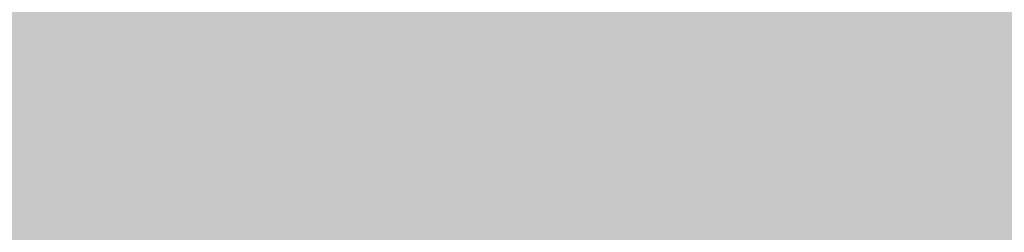
# Model space of a CAD drawing. Units: millimetres. Extents: x -22994 to 29398, y -19990 to 20176.
# Tile 75 of 135: x 226.355 to 227.437, y 84.264 to 84.498. Entities that reach past the tile are written whole.
import ezdxf
from ezdxf import colors
from ezdxf.entities.mleader import LeaderData, LeaderLine
from ezdxf.math import Vec2, Vec3

# ---------------------------------------------------------------- set-up
doc = ezdxf.new("R2010")
doc.units = ezdxf.units.MM
doc.header["$MEASUREMENT"] = 0
for name, color, linetype, lineweight in [('M-ANNO-TEXT', 7, 'Continuous', 25), ('M-DIMS', 2, 'Continuous', 18), ('M-EQPM-PATT', 7, 'Continuous', 18)]:
    doc.layers.add(name, color=color, linetype=linetype, lineweight=lineweight)
doc.styles.get("Standard").update_dxf_attribs({"font": 'arial.ttf'})
doc.dimstyles.get("Standard").update_dxf_attribs({"dimtxt": 0.18, "dimasz": 10000, "dimexe": 0.18, "dimexo": 0.0625, "dimgap": 0.09, "dimtad": 0, "dimtih": 1, "dimtoh": 1, "dimdec": 0, "dimzin": 0, "dimdsep": 46, "dimtxsty": 'Standard', "dimcen": 0.09, "dimadec": 0, "dimazin": 0, "dimtfac": 1, "dimtdec": 0, "dimtofl": 0, "dimtmove": 0, "dimatfit": 3, "dimfxl": 1, "dimtolj": 1, "dimtzin": 0, "dimlwd": 30, "dimarcsym": 0})

# ---------------------------------------------------------------- blocks, each defined once
blk = doc.blocks.new('*D2')
at = {"layer": 'Defpoints', "color": 0, "transparency": 16777216}
for p in [(6.6773, 10.2713), (290.852, 10.2713), (290.852, -5.0787)]:
    blk.add_point(p, dxfattribs=at)
at = {"layer": 'M-DIMS', "color": 0, "lineweight": -2, "transparency": 16777216}
for p, q in [((6.6773, 10.2088), (6.6773, -5.2587)), ((290.852, 10.2088), (290.852, -5.2587))]:
    blk.add_line(p, q, dxfattribs=at)
at = {"layer": 'M-DIMS', "color": 0, "lineweight": 30, "transparency": 16777216}
for p, q in [((-9993.3227, -5.0787), (-19993.3227, -5.0787)), ((10290.852, -5.0787), (20290.852, -5.0787))]:
    blk.add_line(p, q, dxfattribs=at)
at = {"layer": 'M-DIMS', "color": 0, "transparency": 16777216}
for points in [[(-9993.3227, 1661.5879), (-9993.3227, -1671.7454), (6.6773, -5.0787)], [(10290.852, 1661.5879), (10290.852, -1671.7454), (290.852, -5.0787)]]:
    blk.add_solid(points, dxfattribs=at)
at = {"layer": 'M-DIMS', "color": 0, "transparency": 16777216, "insert": (148.7647, -5.0787), "char_height": 0.18, "attachment_point": 5}
blk.add_mtext('\\A1;284.2', dxfattribs=at)
blk = doc.blocks.new('*D3')
at = {"layer": 'Defpoints', "color": 0, "transparency": 16777216}
for p in [(110.2647, 204.1654), (110.2647, 176.3662), (95.8327, 127.967)]:
    blk.add_point(p, dxfattribs=at)
at = {"layer": 'M-DIMS', "color": 0, "lineweight": -2, "transparency": 16777216}
for p, q in [((95.8327, 128.0295), (95.8327, 204.3454)), ((110.2647, 176.4287), (110.2647, 204.3454))]:
    blk.add_line(p, q, dxfattribs=at)
at = {"layer": 'M-DIMS', "color": 0, "lineweight": 30, "transparency": 16777216}
for p, q in [((-9904.1673, 204.1654), (-19904.1673, 204.1654)), ((10110.2647, 204.1654), (20110.2647, 204.1654))]:
    blk.add_line(p, q, dxfattribs=at)
at = {"layer": 'M-DIMS', "color": 0, "transparency": 16777216}
for points in [[(-9904.1673, 1870.8321), (-9904.1673, -1462.5013), (95.8327, 204.1654)], [(10110.2647, 1870.8321), (10110.2647, -1462.5013), (110.2647, 204.1654)]]:
    blk.add_solid(points, dxfattribs=at)
at = {"layer": 'M-DIMS', "color": 0, "transparency": 16777216, "insert": (103.0487, 204.1654), "char_height": 0.18, "attachment_point": 5}
blk.add_mtext('\\A1;14.432', dxfattribs=at)
blk = doc.blocks.new('*D4')
at = {"layer": 'Defpoints', "color": 0, "transparency": 16777216}
for p in [(116.2647, 204.1654), (110.2647, 176.3662), (116.2647, 176.3662)]:
    blk.add_point(p, dxfattribs=at)
at = {"layer": 'M-DIMS', "color": 0, "lineweight": -2, "transparency": 16777216}
for p, q in [((110.2647, 176.4287), (110.2647, 204.3454)), ((116.2647, 176.4287), (116.2647, 204.3454))]:
    blk.add_line(p, q, dxfattribs=at)
at = {"layer": 'M-DIMS', "color": 0, "lineweight": 30, "transparency": 16777216}
for p, q in [((-9889.7353, 204.1654), (-19889.7353, 204.1654)), ((10116.2647, 204.1654), (20116.2647, 204.1654))]:
    blk.add_line(p, q, dxfattribs=at)
at = {"layer": 'M-DIMS', "color": 0, "transparency": 16777216}
for points in [[(-9889.7353, 1870.8321), (-9889.7353, -1462.5013), (110.2647, 204.1654)], [(10116.2647, 1870.8321), (10116.2647, -1462.5013), (116.2647, 204.1654)]]:
    blk.add_solid(points, dxfattribs=at)
at = {"layer": 'M-DIMS', "color": 0, "transparency": 16777216, "insert": (113.2647, 204.1654), "char_height": 0.18, "attachment_point": 5}
blk.add_mtext('\\A1;6', dxfattribs=at)
blk = doc.blocks.new('*D5')
at = {"layer": 'Defpoints', "color": 0, "transparency": 16777216}
for p in [(181.2647, 204.1654), (116.2647, 176.3662), (181.2647, 176.3662)]:
    blk.add_point(p, dxfattribs=at)
at = {"layer": 'M-DIMS', "color": 0, "lineweight": -2, "transparency": 16777216}
for p, q in [((116.2647, 176.4287), (116.2647, 204.3454)), ((181.2647, 176.4287), (181.2647, 204.3454))]:
    blk.add_line(p, q, dxfattribs=at)
at = {"layer": 'M-DIMS', "color": 0, "lineweight": 30, "transparency": 16777216}
for p, q in [((-9883.7353, 204.1654), (-19883.7353, 204.1654)), ((10181.2647, 204.1654), (20181.2647, 204.1654))]:
    blk.add_line(p, q, dxfattribs=at)
at = {"layer": 'M-DIMS', "color": 0, "transparency": 16777216}
for points in [[(-9883.7353, 1870.8321), (-9883.7353, -1462.5013), (116.2647, 204.1654)], [(10181.2647, 1870.8321), (10181.2647, -1462.5013), (181.2647, 204.1654)]]:
    blk.add_solid(points, dxfattribs=at)
at = {"layer": 'M-DIMS', "color": 0, "transparency": 16777216, "insert": (148.7647, 204.1654), "char_height": 0.18, "attachment_point": 5}
blk.add_mtext('\\A1;65', dxfattribs=at)
blk = doc.blocks.new('*D6')
at = {"layer": 'Defpoints', "color": 0, "transparency": 16777216}
for p in [(187.2647, 204.1654), (181.2647, 176.3662), (187.2647, 176.3662)]:
    blk.add_point(p, dxfattribs=at)
at = {"layer": 'M-DIMS', "color": 0, "lineweight": -2, "transparency": 16777216}
for p, q in [((181.2647, 176.4287), (181.2647, 204.3454)), ((187.2647, 176.4287), (187.2647, 204.3454))]:
    blk.add_line(p, q, dxfattribs=at)
at = {"layer": 'M-DIMS', "color": 0, "lineweight": 30, "transparency": 16777216}
for p, q in [((-9818.7353, 204.1654), (-19818.7353, 204.1654)), ((10187.2647, 204.1654), (20187.2647, 204.1654))]:
    blk.add_line(p, q, dxfattribs=at)
at = {"layer": 'M-DIMS', "color": 0, "transparency": 16777216}
for points in [[(-9818.7353, 1870.8321), (-9818.7353, -1462.5013), (181.2647, 204.1654)], [(10187.2647, 1870.8321), (10187.2647, -1462.5013), (187.2647, 204.1654)]]:
    blk.add_solid(points, dxfattribs=at)
at = {"layer": 'M-DIMS', "color": 0, "transparency": 16777216, "insert": (184.2647, 204.1654), "char_height": 0.18, "attachment_point": 5}
blk.add_mtext('\\A1;6', dxfattribs=at)
blk = doc.blocks.new('*D7')
at = {"layer": 'Defpoints', "color": 0, "transparency": 16777216}
for p in [(201.6967, 204.1654), (187.2647, 176.3662), (201.6967, 127.967)]:
    blk.add_point(p, dxfattribs=at)
at = {"layer": 'M-DIMS', "color": 0, "lineweight": -2, "transparency": 16777216}
for p, q in [((187.2647, 176.4287), (187.2647, 204.3454)), ((201.6967, 128.0295), (201.6967, 204.3454))]:
    blk.add_line(p, q, dxfattribs=at)
at = {"layer": 'M-DIMS', "color": 0, "lineweight": 30, "transparency": 16777216}
for p, q in [((-9812.7353, 204.1654), (-19812.7353, 204.1654)), ((10201.6967, 204.1654), (20201.6967, 204.1654))]:
    blk.add_line(p, q, dxfattribs=at)
at = {"layer": 'M-DIMS', "color": 0, "transparency": 16777216}
for points in [[(-9812.7353, 1870.8321), (-9812.7353, -1462.5013), (187.2647, 204.1654)], [(10201.6967, 1870.8321), (10201.6967, -1462.5013), (201.6967, 204.1654)]]:
    blk.add_solid(points, dxfattribs=at)
at = {"layer": 'M-DIMS', "color": 0, "transparency": 16777216, "insert": (194.4807, 204.1654), "char_height": 0.18, "attachment_point": 5}
blk.add_mtext('\\A1;14.432', dxfattribs=at)
blk = doc.blocks.new('*D8')
at = {"layer": 'Defpoints', "color": 0, "transparency": 16777216}
for p in [(227.6485, 204.1654), (227.6485, 146.7296), (201.6967, 127.967)]:
    blk.add_point(p, dxfattribs=at)
at = {"layer": 'M-DIMS', "color": 0, "lineweight": -2, "transparency": 16777216}
for p, q in [((201.6967, 128.0295), (201.6967, 204.3454)), ((227.6485, 146.7921), (227.6485, 204.3454))]:
    blk.add_line(p, q, dxfattribs=at)
at = {"layer": 'M-DIMS', "color": 0, "lineweight": 30, "transparency": 16777216}
for p, q in [((-9798.3033, 204.1654), (-19798.3033, 204.1654)), ((10227.6485, 204.1654), (20227.6485, 204.1654))]:
    blk.add_line(p, q, dxfattribs=at)
at = {"layer": 'M-DIMS', "color": 0, "transparency": 16777216}
for points in [[(-9798.3033, 1870.8321), (-9798.3033, -1462.5013), (201.6967, 204.1654)], [(10227.6485, 1870.8321), (10227.6485, -1462.5013), (227.6485, 204.1654)]]:
    blk.add_solid(points, dxfattribs=at)
at = {"layer": 'M-DIMS', "color": 0, "transparency": 16777216, "insert": (214.6726, 204.1654), "char_height": 0.18, "attachment_point": 5}
blk.add_mtext('\\A1;25.95', dxfattribs=at)
blk = doc.blocks.new('*D9')
at = {"layer": 'Defpoints', "color": 0, "transparency": 16777216}
for p in [(187.2647, 176.3662), (306.202, 176.3662), (290.852, 10.2713)]:
    blk.add_point(p, dxfattribs=at)
at = {"layer": 'M-DIMS', "color": 0, "lineweight": 30, "transparency": 16777216}
for p, q in [((306.202, 10176.3662), (306.202, 20176.3662)), ((306.202, -9989.7287), (306.202, -19989.7287))]:
    blk.add_line(p, q, dxfattribs=at)
at = {"layer": 'M-DIMS', "color": 0, "lineweight": -2, "transparency": 16777216}
for p, q in [((187.3272, 176.3662), (306.382, 176.3662)), ((290.9145, 10.2713), (306.382, 10.2713))]:
    blk.add_line(p, q, dxfattribs=at)
at = {"layer": 'M-DIMS', "color": 0, "transparency": 16777216}
for points in [[(-1360.4646, 10176.3662), (1972.8687, 10176.3662), (306.202, 176.3662)], [(-1360.4646, -9989.7287), (1972.8687, -9989.7287), (306.202, 10.2713)]]:
    blk.add_solid(points, dxfattribs=at)
at = {"layer": 'M-DIMS', "color": 0, "transparency": 16777216, "insert": (306.202, 93.3187), "char_height": 0.18, "attachment_point": 5}
blk.add_mtext('\\A1;166.1', dxfattribs=at)
blk = doc.blocks.new('*D10')
at = {"layer": 'Defpoints', "color": 0, "transparency": 16777216}
for p in [(125.6498, 136.0713), (133.3459, 136.0713), (133.3459, -5.0787)]:
    blk.add_point(p, dxfattribs=at)
at = {"layer": 'M-DIMS', "color": 0, "lineweight": -2, "transparency": 16777216}
for p, q in [((125.6498, 136.0088), (125.6498, -5.2587)), ((133.3459, 136.0088), (133.3459, -5.2587))]:
    blk.add_line(p, q, dxfattribs=at)
at = {"layer": 'M-DIMS', "color": 0, "lineweight": 30, "transparency": 16777216}
for p, q in [((-9874.3502, -5.0787), (-19874.3502, -5.0787)), ((10133.3459, -5.0787), (20133.3459, -5.0787))]:
    blk.add_line(p, q, dxfattribs=at)
at = {"layer": 'M-DIMS', "color": 0, "transparency": 16777216}
for points in [[(-9874.3502, 1661.5879), (-9874.3502, -1671.7454), (125.6498, -5.0787)], [(10133.3459, 1661.5879), (10133.3459, -1671.7454), (133.3459, -5.0787)]]:
    blk.add_solid(points, dxfattribs=at)
at = {"layer": 'M-DIMS', "color": 0, "transparency": 16777216, "insert": (129.4978, -5.0787), "char_height": 0.18, "attachment_point": 5}
blk.add_mtext('\\A1;7.696', dxfattribs=at)
blk = doc.blocks.new('*D11')
at = {"layer": 'Defpoints', "color": 0, "transparency": 16777216}
for p in [(133.3459, 136.0713), (135.6498, 136.0713), (135.6498, -5.0787)]:
    blk.add_point(p, dxfattribs=at)
at = {"layer": 'M-DIMS', "color": 0, "lineweight": -2, "transparency": 16777216}
for p, q in [((133.3459, 136.0088), (133.3459, -5.2587)), ((135.6498, 136.0088), (135.6498, -5.2587))]:
    blk.add_line(p, q, dxfattribs=at)
at = {"layer": 'M-DIMS', "color": 0, "lineweight": 30, "transparency": 16777216}
for p, q in [((-9866.6541, -5.0787), (-19866.6541, -5.0787)), ((10135.6498, -5.0787), (20135.6498, -5.0787))]:
    blk.add_line(p, q, dxfattribs=at)
at = {"layer": 'M-DIMS', "color": 0, "transparency": 16777216}
for points in [[(-9866.6541, 1661.5879), (-9866.6541, -1671.7454), (133.3459, -5.0787)], [(10135.6498, 1661.5879), (10135.6498, -1671.7454), (135.6498, -5.0787)]]:
    blk.add_solid(points, dxfattribs=at)
at = {"layer": 'M-DIMS', "color": 0, "transparency": 16777216, "insert": (134.4978, -5.0787), "char_height": 0.18, "attachment_point": 5}
blk.add_mtext('\\A1;2.304', dxfattribs=at)
blk = doc.blocks.new('*D12')
at = {"layer": 'Defpoints', "color": 0, "transparency": 16777216}
for p in [(135.6498, 136.0713), (145.6498, 136.0713), (145.6498, -5.0787)]:
    blk.add_point(p, dxfattribs=at)
at = {"layer": 'M-DIMS', "color": 0, "lineweight": -2, "transparency": 16777216}
for p, q in [((135.6498, 136.0088), (135.6498, -5.2587)), ((145.6498, 136.0088), (145.6498, -5.2587))]:
    blk.add_line(p, q, dxfattribs=at)
at = {"layer": 'M-DIMS', "color": 0, "lineweight": 30, "transparency": 16777216}
for p, q in [((-9864.3502, -5.0787), (-19864.3502, -5.0787)), ((10145.6498, -5.0787), (20145.6498, -5.0787))]:
    blk.add_line(p, q, dxfattribs=at)
at = {"layer": 'M-DIMS', "color": 0, "transparency": 16777216}
for points in [[(-9864.3502, 1661.5879), (-9864.3502, -1671.7454), (135.6498, -5.0787)], [(10145.6498, 1661.5879), (10145.6498, -1671.7454), (145.6498, -5.0787)]]:
    blk.add_solid(points, dxfattribs=at)
at = {"layer": 'M-DIMS', "color": 0, "transparency": 16777216, "insert": (140.6498, -5.0787), "char_height": 0.18, "attachment_point": 5}
blk.add_mtext('\\A1;10', dxfattribs=at)
blk = doc.blocks.new('*D13')
at = {"layer": 'Defpoints', "color": 0, "transparency": 16777216}
for p in [(145.6498, 136.0713), (155.6498, 136.0713), (155.6498, -5.0787)]:
    blk.add_point(p, dxfattribs=at)
at = {"layer": 'M-DIMS', "color": 0, "lineweight": -2, "transparency": 16777216}
for p, q in [((145.6498, 136.0088), (145.6498, -5.2587)), ((155.6498, 136.0088), (155.6498, -5.2587))]:
    blk.add_line(p, q, dxfattribs=at)
at = {"layer": 'M-DIMS', "color": 0, "lineweight": 30, "transparency": 16777216}
for p, q in [((-9854.3502, -5.0787), (-19854.3502, -5.0787)), ((10155.6498, -5.0787), (20155.6498, -5.0787))]:
    blk.add_line(p, q, dxfattribs=at)
at = {"layer": 'M-DIMS', "color": 0, "transparency": 16777216}
for points in [[(-9854.3502, 1661.5879), (-9854.3502, -1671.7454), (145.6498, -5.0787)], [(10155.6498, 1661.5879), (10155.6498, -1671.7454), (155.6498, -5.0787)]]:
    blk.add_solid(points, dxfattribs=at)
at = {"layer": 'M-DIMS', "color": 0, "transparency": 16777216, "insert": (150.6498, -5.0787), "char_height": 0.18, "attachment_point": 5}
blk.add_mtext('\\A1;10', dxfattribs=at)
blk = doc.blocks.new('*D14')
at = {"layer": 'Defpoints', "color": 0, "transparency": 16777216}
for p in [(155.6498, 136.0713), (165.6498, 136.0713), (165.6498, -5.0787)]:
    blk.add_point(p, dxfattribs=at)
at = {"layer": 'M-DIMS', "color": 0, "lineweight": -2, "transparency": 16777216}
for p, q in [((155.6498, 136.0088), (155.6498, -5.2587)), ((165.6498, 136.0088), (165.6498, -5.2587))]:
    blk.add_line(p, q, dxfattribs=at)
at = {"layer": 'M-DIMS', "color": 0, "lineweight": 30, "transparency": 16777216}
for p, q in [((-9844.3502, -5.0787), (-19844.3502, -5.0787)), ((10165.6498, -5.0787), (20165.6498, -5.0787))]:
    blk.add_line(p, q, dxfattribs=at)
at = {"layer": 'M-DIMS', "color": 0, "transparency": 16777216}
for points in [[(-9844.3502, 1661.5879), (-9844.3502, -1671.7454), (155.6498, -5.0787)], [(10165.6498, 1661.5879), (10165.6498, -1671.7454), (165.6498, -5.0787)]]:
    blk.add_solid(points, dxfattribs=at)
at = {"layer": 'M-DIMS', "color": 0, "transparency": 16777216, "insert": (160.6498, -5.0787), "char_height": 0.18, "attachment_point": 5}
blk.add_mtext('\\A1;10', dxfattribs=at)
blk = doc.blocks.new('*D15')
at = {"layer": 'Defpoints', "color": 0, "transparency": 16777216}
for p in [(173.3459, 154.788), (173.3459, 136.0713), (306.202, 136.0713)]:
    blk.add_point(p, dxfattribs=at)
at = {"layer": 'M-DIMS', "color": 0, "lineweight": 30, "transparency": 16777216}
for p, q in [((306.202, 10154.788), (306.202, 20154.788)), ((306.202, -9863.9287), (306.202, -19863.9287))]:
    blk.add_line(p, q, dxfattribs=at)
at = {"layer": 'M-DIMS', "color": 0, "lineweight": -2, "transparency": 16777216}
for p, q in [((173.4084, 154.788), (306.382, 154.788)), ((173.4084, 136.0713), (306.382, 136.0713))]:
    blk.add_line(p, q, dxfattribs=at)
at = {"layer": 'M-DIMS', "color": 0, "transparency": 16777216}
for points in [[(-1360.4646, 10154.788), (1972.8687, 10154.788), (306.202, 154.788)], [(-1360.4646, -9863.9287), (1972.8687, -9863.9287), (306.202, 136.0713)]]:
    blk.add_solid(points, dxfattribs=at)
at = {"layer": 'M-DIMS', "color": 0, "transparency": 16777216, "insert": (306.202, 145.4297), "char_height": 0.18, "attachment_point": 5}
blk.add_mtext('\\A1;18.717', dxfattribs=at)
blk = doc.blocks.new('*D16')
at = {"layer": 'Defpoints', "color": 0, "transparency": 16777216}
for p in [(120.1702, 204.1654), (110.4658, 48.0349), (120.1702, 48.0349)]:
    blk.add_point(p, dxfattribs=at)
at = {"layer": 'M-DIMS', "color": 0, "lineweight": -2, "transparency": 16777216}
for p, q in [((110.4658, 48.0974), (110.4658, 204.3454)), ((120.1702, 48.0974), (120.1702, 204.3454))]:
    blk.add_line(p, q, dxfattribs=at)
at = {"layer": 'M-DIMS', "color": 0, "lineweight": 30, "transparency": 16777216}
for p, q in [((-9889.5342, 204.1654), (-19889.5342, 204.1654)), ((10120.1702, 204.1654), (20120.1702, 204.1654))]:
    blk.add_line(p, q, dxfattribs=at)
at = {"layer": 'M-DIMS', "color": 0, "transparency": 16777216}
for points in [[(-9889.5342, 1870.8321), (-9889.5342, -1462.5013), (110.4658, 204.1654)], [(10120.1702, 1870.8321), (10120.1702, -1462.5013), (120.1702, 204.1654)]]:
    blk.add_solid(points, dxfattribs=at)
at = {"layer": 'M-DIMS', "color": 0, "transparency": 16777216, "insert": (115.318, 204.1654), "char_height": 0.18, "attachment_point": 5}
blk.add_mtext('\\A1;9.704', dxfattribs=at)
blk = doc.blocks.new('*D17')
at = {"layer": 'Defpoints', "color": 0, "transparency": 16777216}
for p in [(126.1702, 204.1654), (120.1702, 48.0349), (126.1702, 48.0349)]:
    blk.add_point(p, dxfattribs=at)
at = {"layer": 'M-DIMS', "color": 0, "lineweight": -2, "transparency": 16777216}
for p, q in [((120.1702, 48.0974), (120.1702, 204.3454)), ((126.1702, 48.0974), (126.1702, 204.3454))]:
    blk.add_line(p, q, dxfattribs=at)
at = {"layer": 'M-DIMS', "color": 0, "lineweight": 30, "transparency": 16777216}
for p, q in [((-9879.8298, 204.1654), (-19879.8298, 204.1654)), ((10126.1702, 204.1654), (20126.1702, 204.1654))]:
    blk.add_line(p, q, dxfattribs=at)
at = {"layer": 'M-DIMS', "color": 0, "transparency": 16777216}
for points in [[(-9879.8298, 1870.8321), (-9879.8298, -1462.5013), (120.1702, 204.1654)], [(10126.1702, 1870.8321), (10126.1702, -1462.5013), (126.1702, 204.1654)]]:
    blk.add_solid(points, dxfattribs=at)
at = {"layer": 'M-DIMS', "color": 0, "transparency": 16777216, "insert": (123.1702, 204.1654), "char_height": 0.18, "attachment_point": 5}
blk.add_mtext('\\A1;6', dxfattribs=at)
blk = doc.blocks.new('*D18')
at = {"layer": 'Defpoints', "color": 0, "transparency": 16777216}
for p in [(132.1702, 204.1654), (126.1702, 48.0349), (132.1702, 48.0349)]:
    blk.add_point(p, dxfattribs=at)
at = {"layer": 'M-DIMS', "color": 0, "lineweight": -2, "transparency": 16777216}
for p, q in [((126.1702, 48.0974), (126.1702, 204.3454)), ((132.1702, 48.0974), (132.1702, 204.3454))]:
    blk.add_line(p, q, dxfattribs=at)
at = {"layer": 'M-DIMS', "color": 0, "lineweight": 30, "transparency": 16777216}
for p, q in [((-9873.8298, 204.1654), (-19873.8298, 204.1654)), ((10132.1702, 204.1654), (20132.1702, 204.1654))]:
    blk.add_line(p, q, dxfattribs=at)
at = {"layer": 'M-DIMS', "color": 0, "transparency": 16777216}
for points in [[(-9873.8298, 1870.8321), (-9873.8298, -1462.5013), (126.1702, 204.1654)], [(10132.1702, 1870.8321), (10132.1702, -1462.5013), (132.1702, 204.1654)]]:
    blk.add_solid(points, dxfattribs=at)
at = {"layer": 'M-DIMS', "color": 0, "transparency": 16777216, "insert": (129.1702, 204.1654), "char_height": 0.18, "attachment_point": 5}
blk.add_mtext('\\A1;6', dxfattribs=at)
blk = doc.blocks.new('*D19')
at = {"layer": 'Defpoints', "color": 0, "transparency": 16777216}
for p in [(138.1702, 204.1654), (132.1702, 48.0349), (138.1702, 48.0349)]:
    blk.add_point(p, dxfattribs=at)
at = {"layer": 'M-DIMS', "color": 0, "lineweight": -2, "transparency": 16777216}
for p, q in [((132.1702, 48.0974), (132.1702, 204.3454)), ((138.1702, 48.0974), (138.1702, 204.3454))]:
    blk.add_line(p, q, dxfattribs=at)
at = {"layer": 'M-DIMS', "color": 0, "lineweight": 30, "transparency": 16777216}
for p, q in [((-9867.8298, 204.1654), (-19867.8298, 204.1654)), ((10138.1702, 204.1654), (20138.1702, 204.1654))]:
    blk.add_line(p, q, dxfattribs=at)
at = {"layer": 'M-DIMS', "color": 0, "transparency": 16777216}
for points in [[(-9867.8298, 1870.8321), (-9867.8298, -1462.5013), (132.1702, 204.1654)], [(10138.1702, 1870.8321), (10138.1702, -1462.5013), (138.1702, 204.1654)]]:
    blk.add_solid(points, dxfattribs=at)
at = {"layer": 'M-DIMS', "color": 0, "transparency": 16777216, "insert": (135.1702, 204.1654), "char_height": 0.18, "attachment_point": 5}
blk.add_mtext('\\A1;6', dxfattribs=at)
blk = doc.blocks.new('*D20')
at = {"layer": 'Defpoints', "color": 0, "transparency": 16777216}
for p in [(144.1702, 204.1654), (138.1702, 48.0349), (144.1702, 48.0349)]:
    blk.add_point(p, dxfattribs=at)
at = {"layer": 'M-DIMS', "color": 0, "lineweight": -2, "transparency": 16777216}
for p, q in [((138.1702, 48.0974), (138.1702, 204.3454)), ((144.1702, 48.0974), (144.1702, 204.3454))]:
    blk.add_line(p, q, dxfattribs=at)
at = {"layer": 'M-DIMS', "color": 0, "lineweight": 30, "transparency": 16777216}
for p, q in [((-9861.8298, 204.1654), (-19861.8298, 204.1654)), ((10144.1702, 204.1654), (20144.1702, 204.1654))]:
    blk.add_line(p, q, dxfattribs=at)
at = {"layer": 'M-DIMS', "color": 0, "transparency": 16777216}
for points in [[(-9861.8298, 1870.8321), (-9861.8298, -1462.5013), (138.1702, 204.1654)], [(10144.1702, 1870.8321), (10144.1702, -1462.5013), (144.1702, 204.1654)]]:
    blk.add_solid(points, dxfattribs=at)
at = {"layer": 'M-DIMS', "color": 0, "transparency": 16777216, "insert": (141.1702, 204.1654), "char_height": 0.18, "attachment_point": 5}
blk.add_mtext('\\A1;6', dxfattribs=at)
blk = doc.blocks.new('*D21')
at = {"layer": 'Defpoints', "color": 0, "transparency": 16777216}
for p in [(149.1157, 204.1654), (144.1702, 48.0349), (149.1157, 48.0349)]:
    blk.add_point(p, dxfattribs=at)
at = {"layer": 'M-DIMS', "color": 0, "lineweight": -2, "transparency": 16777216}
for p, q in [((144.1702, 48.0974), (144.1702, 204.3454)), ((149.1157, 48.0974), (149.1157, 204.3454))]:
    blk.add_line(p, q, dxfattribs=at)
at = {"layer": 'M-DIMS', "color": 0, "lineweight": 30, "transparency": 16777216}
for p, q in [((-9855.8298, 204.1654), (-19855.8298, 204.1654)), ((10149.1157, 204.1654), (20149.1157, 204.1654))]:
    blk.add_line(p, q, dxfattribs=at)
at = {"layer": 'M-DIMS', "color": 0, "transparency": 16777216}
for points in [[(-9855.8298, 1870.8321), (-9855.8298, -1462.5013), (144.1702, 204.1654)], [(10149.1157, 1870.8321), (10149.1157, -1462.5013), (149.1157, 204.1654)]]:
    blk.add_solid(points, dxfattribs=at)
at = {"layer": 'M-DIMS', "color": 0, "transparency": 16777216, "insert": (146.6429, 204.1654), "char_height": 0.18, "attachment_point": 5}
blk.add_mtext('\\A1;4.945', dxfattribs=at)
blk = doc.blocks.new('*D22')
at = {"layer": 'Defpoints', "color": 0, "transparency": 16777216}
for p in [(149.1157, 30.9895), (155.1157, 30.9895), (155.1157, -5.0787)]:
    blk.add_point(p, dxfattribs=at)
at = {"layer": 'M-DIMS', "color": 0, "lineweight": -2, "transparency": 16777216}
for p, q in [((149.1157, 30.927), (149.1157, -5.2587)), ((155.1157, 30.927), (155.1157, -5.2587))]:
    blk.add_line(p, q, dxfattribs=at)
at = {"layer": 'M-DIMS', "color": 0, "lineweight": 30, "transparency": 16777216}
for p, q in [((-9850.8843, -5.0787), (-19850.8843, -5.0787)), ((10155.1157, -5.0787), (20155.1157, -5.0787))]:
    blk.add_line(p, q, dxfattribs=at)
at = {"layer": 'M-DIMS', "color": 0, "transparency": 16777216}
for points in [[(-9850.8843, 1661.5879), (-9850.8843, -1671.7454), (149.1157, -5.0787)], [(10155.1157, 1661.5879), (10155.1157, -1671.7454), (155.1157, -5.0787)]]:
    blk.add_solid(points, dxfattribs=at)
at = {"layer": 'M-DIMS', "color": 0, "transparency": 16777216, "insert": (152.1157, -5.0787), "char_height": 0.18, "attachment_point": 5}
blk.add_mtext('\\A1;6', dxfattribs=at)
blk = doc.blocks.new('*D23')
at = {"layer": 'Defpoints', "color": 0, "transparency": 16777216}
for p in [(155.1157, 30.9895), (161.1157, 30.9895), (161.1157, -5.0787)]:
    blk.add_point(p, dxfattribs=at)
at = {"layer": 'M-DIMS', "color": 0, "lineweight": -2, "transparency": 16777216}
for p, q in [((155.1157, 30.927), (155.1157, -5.2587)), ((161.1157, 30.927), (161.1157, -5.2587))]:
    blk.add_line(p, q, dxfattribs=at)
at = {"layer": 'M-DIMS', "color": 0, "lineweight": 30, "transparency": 16777216}
for p, q in [((-9844.8843, -5.0787), (-19844.8843, -5.0787)), ((10161.1157, -5.0787), (20161.1157, -5.0787))]:
    blk.add_line(p, q, dxfattribs=at)
at = {"layer": 'M-DIMS', "color": 0, "transparency": 16777216}
for points in [[(-9844.8843, 1661.5879), (-9844.8843, -1671.7454), (155.1157, -5.0787)], [(10161.1157, 1661.5879), (10161.1157, -1671.7454), (161.1157, -5.0787)]]:
    blk.add_solid(points, dxfattribs=at)
at = {"layer": 'M-DIMS', "color": 0, "transparency": 16777216, "insert": (158.1157, -5.0787), "char_height": 0.18, "attachment_point": 5}
blk.add_mtext('\\A1;6', dxfattribs=at)
blk = doc.blocks.new('*D24')
at = {"layer": 'Defpoints', "color": 0, "transparency": 16777216}
for p in [(161.1157, 30.9895), (166.4387, 30.9895), (166.4387, -5.0787)]:
    blk.add_point(p, dxfattribs=at)
at = {"layer": 'M-DIMS', "color": 0, "lineweight": -2, "transparency": 16777216}
for p, q in [((161.1157, 30.927), (161.1157, -5.2587)), ((166.4387, 30.927), (166.4387, -5.2587))]:
    blk.add_line(p, q, dxfattribs=at)
at = {"layer": 'M-DIMS', "color": 0, "lineweight": 30, "transparency": 16777216}
for p, q in [((-9838.8843, -5.0787), (-19838.8843, -5.0787)), ((10166.4387, -5.0787), (20166.4387, -5.0787))]:
    blk.add_line(p, q, dxfattribs=at)
at = {"layer": 'M-DIMS', "color": 0, "transparency": 16777216}
for points in [[(-9838.8843, 1661.5879), (-9838.8843, -1671.7454), (161.1157, -5.0787)], [(10166.4387, 1661.5879), (10166.4387, -1671.7454), (166.4387, -5.0787)]]:
    blk.add_solid(points, dxfattribs=at)
at = {"layer": 'M-DIMS', "color": 0, "transparency": 16777216, "insert": (163.7772, -5.0787), "char_height": 0.18, "attachment_point": 5}
blk.add_mtext('\\A1;5.323', dxfattribs=at)
blk = doc.blocks.new('*D25')
at = {"layer": 'Defpoints', "color": 0, "transparency": 16777216}
for p in [(166.4387, 30.9895), (172.4387, 30.9895), (172.4387, -5.0787)]:
    blk.add_point(p, dxfattribs=at)
at = {"layer": 'M-DIMS', "color": 0, "lineweight": -2, "transparency": 16777216}
for p, q in [((166.4387, 30.927), (166.4387, -5.2587)), ((172.4387, 30.927), (172.4387, -5.2587))]:
    blk.add_line(p, q, dxfattribs=at)
at = {"layer": 'M-DIMS', "color": 0, "lineweight": 30, "transparency": 16777216}
for p, q in [((-9833.5613, -5.0787), (-19833.5613, -5.0787)), ((10172.4387, -5.0787), (20172.4387, -5.0787))]:
    blk.add_line(p, q, dxfattribs=at)
at = {"layer": 'M-DIMS', "color": 0, "transparency": 16777216}
for points in [[(-9833.5613, 1661.5879), (-9833.5613, -1671.7454), (166.4387, -5.0787)], [(10172.4387, 1661.5879), (10172.4387, -1671.7454), (172.4387, -5.0787)]]:
    blk.add_solid(points, dxfattribs=at)
at = {"layer": 'M-DIMS', "color": 0, "transparency": 16777216, "insert": (169.4387, -5.0787), "char_height": 0.18, "attachment_point": 5}
blk.add_mtext('\\A1;6', dxfattribs=at)
blk = doc.blocks.new('*D26')
at = {"layer": 'Defpoints', "color": 0, "transparency": 16777216}
for p in [(172.4387, 30.9895), (178.4387, 30.9895), (178.4387, -5.0787)]:
    blk.add_point(p, dxfattribs=at)
at = {"layer": 'M-DIMS', "color": 0, "lineweight": -2, "transparency": 16777216}
for p, q in [((172.4387, 30.927), (172.4387, -5.2587)), ((178.4387, 30.927), (178.4387, -5.2587))]:
    blk.add_line(p, q, dxfattribs=at)
at = {"layer": 'M-DIMS', "color": 0, "lineweight": 30, "transparency": 16777216}
for p, q in [((-9827.5613, -5.0787), (-19827.5613, -5.0787)), ((10178.4387, -5.0787), (20178.4387, -5.0787))]:
    blk.add_line(p, q, dxfattribs=at)
at = {"layer": 'M-DIMS', "color": 0, "transparency": 16777216}
for points in [[(-9827.5613, 1661.5879), (-9827.5613, -1671.7454), (172.4387, -5.0787)], [(10178.4387, 1661.5879), (10178.4387, -1671.7454), (178.4387, -5.0787)]]:
    blk.add_solid(points, dxfattribs=at)
at = {"layer": 'M-DIMS', "color": 0, "transparency": 16777216, "insert": (175.4387, -5.0787), "char_height": 0.18, "attachment_point": 5}
blk.add_mtext('\\A1;6', dxfattribs=at)
blk = doc.blocks.new('*D27')
at = {"layer": 'Defpoints', "color": 0, "transparency": 16777216}
for p in [(178.4387, 30.9895), (188.1175, 30.9895), (188.1175, -5.0787)]:
    blk.add_point(p, dxfattribs=at)
at = {"layer": 'M-DIMS', "color": 0, "lineweight": -2, "transparency": 16777216}
for p, q in [((178.4387, 30.927), (178.4387, -5.2587)), ((188.1175, 30.927), (188.1175, -5.2587))]:
    blk.add_line(p, q, dxfattribs=at)
at = {"layer": 'M-DIMS', "color": 0, "lineweight": 30, "transparency": 16777216}
for p, q in [((-9821.5613, -5.0787), (-19821.5613, -5.0787)), ((10188.1175, -5.0787), (20188.1175, -5.0787))]:
    blk.add_line(p, q, dxfattribs=at)
at = {"layer": 'M-DIMS', "color": 0, "transparency": 16777216}
for points in [[(-9821.5613, 1661.5879), (-9821.5613, -1671.7454), (178.4387, -5.0787)], [(10188.1175, 1661.5879), (10188.1175, -1671.7454), (188.1175, -5.0787)]]:
    blk.add_solid(points, dxfattribs=at)
at = {"layer": 'M-DIMS', "color": 0, "transparency": 16777216, "insert": (183.2781, -5.0787), "char_height": 0.18, "attachment_point": 5}
blk.add_mtext('\\A1;9.679', dxfattribs=at)
blk = doc.blocks.new('*D28')
at = {"layer": 'Defpoints', "color": 0, "transparency": 16777216}
for p in [(188.1175, 48.0349), (306.202, 48.0349), (188.1175, 30.9895)]:
    blk.add_point(p, dxfattribs=at)
at = {"layer": 'M-DIMS', "color": 0, "lineweight": 30, "transparency": 16777216}
for p, q in [((306.202, 10048.0349), (306.202, 20048.0349)), ((306.202, -9969.0105), (306.202, -19969.0105))]:
    blk.add_line(p, q, dxfattribs=at)
at = {"layer": 'M-DIMS', "color": 0, "lineweight": -2, "transparency": 16777216}
for p, q in [((188.18, 48.0349), (306.382, 48.0349)), ((188.18, 30.9895), (306.382, 30.9895))]:
    blk.add_line(p, q, dxfattribs=at)
at = {"layer": 'M-DIMS', "color": 0, "transparency": 16777216}
for points in [[(-1360.4646, 10048.0349), (1972.8687, 10048.0349), (306.202, 48.0349)], [(-1360.4646, -9969.0105), (1972.8687, -9969.0105), (306.202, 30.9895)]]:
    blk.add_solid(points, dxfattribs=at)
at = {"layer": 'M-DIMS', "color": 0, "transparency": 16777216, "insert": (306.202, 39.5122), "char_height": 0.18, "attachment_point": 5}
blk.add_mtext('\\A1;17.045', dxfattribs=at)
blk = doc.blocks.new('*D29')
at = {"layer": 'Defpoints', "color": 0, "transparency": 16777216}
for p in [(36.8006, 80.045), (64.0296, 80.045)]:
    blk.add_point(p, dxfattribs=at)
at = {"layer": 'M-DIMS', "color": 0, "lineweight": -2, "transparency": 16777216}
for p, q in [((50.4151, 79.955), (50.4151, 80.135)), ((50.3251, 80.045), (50.5051, 80.045))]:
    blk.add_line(p, q, dxfattribs=at)
at = {"layer": 'M-DIMS', "color": 0, "lineweight": 30, "transparency": 16777216}
blk.add_line((20064.0296, 80.0303), (10064.0296, 80.0377), dxfattribs=at)
at = {"layer": 'M-DIMS', "color": 0, "transparency": 16777216}
blk.add_solid([(10064.0309, 1746.7043), (10064.0284, -1586.629), (64.0296, 80.045)], dxfattribs=at)
at = {"layer": 'M-DIMS', "color": 0, "transparency": 16777216, "insert": (20064.5213, 80.0303), "char_height": 0.18, "attachment_point": 5}
blk.add_mtext('\\A1;∅27.23', dxfattribs=at)
blk = doc.blocks.new('*D30')
at = {"layer": 'Defpoints', "color": 0, "transparency": 16777216}
for p in [(216.3148, 146.7291), (238.9821, 146.73)]:
    blk.add_point(p, dxfattribs=at)
at = {"layer": 'M-DIMS', "color": 0, "lineweight": 30, "transparency": 16777216}
blk.add_line((20238.9821, 147.4959), (10238.9821, 147.1129), dxfattribs=at)
at = {"layer": 'M-DIMS', "color": 0, "lineweight": -2, "transparency": 16777216}
for p, q in [((227.6485, 146.6396), (227.6485, 146.8196)), ((227.5585, 146.7296), (227.7385, 146.7296))]:
    blk.add_line(p, q, dxfattribs=at)
at = {"layer": 'M-DIMS', "color": 0, "transparency": 16777216}
blk.add_solid([(10238.9183, 1813.7796), (10239.0459, -1519.5537), (238.9821, 146.73)], dxfattribs=at)
at = {"layer": 'M-DIMS', "color": 0, "transparency": 16777216, "insert": (20239.5436, 147.4959), "char_height": 0.18, "attachment_point": 5}
blk.add_mtext('\\A1;∅22.667', dxfattribs=at)
blk = doc.blocks.new('*D31')
at = {"layer": 'Defpoints', "color": 0, "transparency": 16777216}
for p in [(223.1641, 146.7291), (232.1328, 146.73)]:
    blk.add_point(p, dxfattribs=at)
at = {"layer": 'M-DIMS', "color": 0, "lineweight": 30, "transparency": 16777216}
blk.add_line((20232.1327, 148.6656), (10232.1328, 147.6978), dxfattribs=at)
at = {"layer": 'M-DIMS', "color": 0, "lineweight": -2, "transparency": 16777216}
for p, q in [((227.6485, 146.6396), (227.6485, 146.8196)), ((227.5585, 146.7296), (227.7385, 146.7296))]:
    blk.add_line(p, q, dxfattribs=at)
at = {"layer": 'M-DIMS', "color": 0, "transparency": 16777216}
blk.add_solid([(10231.9715, 1814.3645), (10232.2941, -1518.9688), (232.1328, 146.73)], dxfattribs=at)
at = {"layer": 'M-DIMS', "color": 0, "transparency": 16777216, "insert": (20232.6245, 148.6656), "char_height": 0.18, "attachment_point": 5}
blk.add_mtext('\\A1;∅8.969', dxfattribs=at)
blk = doc.blocks.new('*D36')
at = {"layer": 'Defpoints', "color": 0, "transparency": 16777216}
for p in [(46.39, 31.3035), (46.3875, 26.5934)]:
    blk.add_point(p, dxfattribs=at)
at = {"layer": 'M-DIMS', "color": 0, "lineweight": 30, "transparency": 16777216}
for p, q in [((57.1499, 20031.3006), (51.77, 10031.302)), ((10057.1499, 20031.3006), (57.1499, 20031.3006))]:
    blk.add_line(p, q, dxfattribs=at)
at = {"layer": 'M-DIMS', "color": 0, "lineweight": -2, "transparency": 16777216}
for p, q in [((46.3887, 28.8585), (46.3887, 29.0385)), ((46.2987, 28.9485), (46.4787, 28.9485))]:
    blk.add_line(p, q, dxfattribs=at)
at = {"layer": 'M-DIMS', "color": 0, "transparency": 16777216}
blk.add_solid([(-1614.8965, 10032.1987), (1718.4364, 10030.4054), (46.39, 31.3035)], dxfattribs=at)
at = {"layer": 'M-DIMS', "color": 0, "transparency": 16777216, "insert": (10057.5542, 20031.3006), "char_height": 0.18, "attachment_point": 5}
blk.add_mtext('\\A1;∅4.71', dxfattribs=at)
blk = doc.blocks.new('*D37')
at = {"layer": 'Defpoints', "color": 0, "transparency": 16777216}
for p in [(54.8343, 118.6145), (59.4936, 118.614)]:
    blk.add_point(p, dxfattribs=at)
at = {"layer": 'M-DIMS', "color": 0, "lineweight": -2, "transparency": 16777216}
for p, q in [((57.1639, 118.5243), (57.1639, 118.7043)), ((57.0739, 118.6143), (57.2539, 118.6143))]:
    blk.add_line(p, q, dxfattribs=at)
at = {"layer": 'M-DIMS', "color": 0, "lineweight": 30, "transparency": 16777216}
blk.add_line((20059.4934, 116.2531), (10059.4935, 117.4336), dxfattribs=at)
at = {"layer": 'M-DIMS', "color": 0, "transparency": 16777216}
blk.add_solid([(10059.6902, 1784.1002), (10059.2968, -1549.2331), (59.4936, 118.614)], dxfattribs=at)
at = {"layer": 'M-DIMS', "color": 0, "transparency": 16777216, "insert": (20059.9852, 116.2531), "char_height": 0.18, "attachment_point": 5}
blk.add_mtext('\\A1;∅4.659', dxfattribs=at)

msp = doc.modelspace()

# ---------------------------------------------------------------- hatches: boundary and pattern name
at = {"layer": 'M-EQPM-PATT'}
h = msp.add_hatch(color=256, dxfattribs=at)
h.set_gradient(color1=(205, 32, 39), color2=(205, 32, 39), tint=1)
h.paths.add_polyline_path([(116.2647, 150.3662), (116.2647, 170.3662), (116.2647, 176.3662), (110.2647, 176.3662), (110.2647, 152.0276), (95.8327, 127.967), (95.8327, 16.6063), (201.6967, 16.6063), (201.6967, 127.967), (187.2647, 152.0276), (187.2647, 176.3662), (181.2647, 176.3662), (181.2647, 170.3662), (181.2647, 150.3662), (195.6967, 126.3055), (195.6967, 22.6063), (101.8327, 22.6063), (101.8327, 126.3055)])
h.paths.add_polyline_path([(185.2208, 88.6347), (101.8327, 88.6347), (101.8327, 87.6347), (182.8066, 87.6347), (178.7313, 83.5594), (195.6967, 83.5594), (195.6967, 84.5594), (181.1455, 84.5594)], flags=17)
h.paths.add_polyline_path([(95.8327, 88.6347), (60.9779, 88.6347, -0.022855), (61.7178, 87.6347), (95.8327, 87.6347)])
h.paths.add_polyline_path([(215.6212, 86.5189), (215.6212, 80.5999), (220.5095, 83.5594)])
h.paths.add_polyline_path([(215.6212, 84.5594), (201.6967, 84.5594), (201.6967, 83.5594), (215.6212, 83.5594)])
h.paths.add_polyline_path([(225.3978, 86.5189), (220.5095, 83.5594), (225.3978, 80.5999)])
h.paths.add_polyline_path([(231.6256, 84.5594), (225.3978, 84.5594), (225.3978, 83.5594), (231.6256, 83.5594)])

# ---------------------------------------------------------------- dimensions: what is measured, and where the dimension line sits
at = {"layer": 'M-DIMS'}
for base, p1, p2, override, picture, middle in [((306.202, 176.3662), (290.852, 10.2713), (187.2647, 176.3662), {"dimdec": 1, "dimlfac": 1, "dimrnd": 0, "dimzin": 0, "dimdsep": 46, "dimlunit": 2}, '*D9', (306.202, 93.3187)), ((306.202, 136.0713), (173.3459, 154.788), (173.3459, 136.0713), {"dimdec": 3, "dimlfac": 1, "dimrnd": 0, "dimzin": 0, "dimdsep": 46, "dimlunit": 2}, '*D15', (306.202, 145.4297)), ((306.202, 48.0349), (188.1175, 30.9895), (188.1175, 48.0349), {"dimdec": 3, "dimlfac": 1, "dimrnd": 0, "dimzin": 0, "dimdsep": 46, "dimlunit": 2}, '*D28', (306.202, 39.5122))]:
    dim = msp.add_linear_dim(base=base, p1=p1, p2=p2, angle=90, dimstyle='Standard', override=override, dxfattribs=at)
    dim.commit()
    dim.dimension.update_dxf_attribs({"geometry": picture, "text_midpoint": middle})
for p1, p2, override, picture, middle in [((46.3875, 26.5934), (46.39, 31.3035), {"dimdec": 2, "dimlfac": 1, "dimrnd": 0, "dimzin": 0, "dimdsep": 46, "dimlunit": 2}, '*D36', (10057.5542, 20031.3006)), ((223.1641, 146.7291), (232.1328, 146.73), {"dimdec": 3, "dimlfac": 1, "dimrnd": 0, "dimzin": 0, "dimdsep": 46, "dimlunit": 2}, '*D31', (20232.1327, 148.6656)), ((216.3148, 146.7291), (238.9821, 146.73), {"dimdec": 3, "dimlfac": 1, "dimrnd": 0, "dimzin": 0, "dimdsep": 46, "dimlunit": 2}, '*D30', (20238.9821, 147.4959))]:
    dim = msp.add_diameter_dim_2p(p1=p1, p2=p2, dimstyle='Standard', override=override, dxfattribs=at)
    dim.commit()
    dim.dimension.update_dxf_attribs({"geometry": picture, "text_midpoint": middle, "dimtype": 163})
for base, p1, p2, override, picture, middle in [((110.2647, 204.1654), (95.8327, 127.967), (110.2647, 176.3662), {"dimdec": 3, "dimlfac": 1, "dimrnd": 0, "dimzin": 0, "dimdsep": 46, "dimlunit": 2}, '*D3', (103.0487, 204.1654)), ((116.2647, 204.1654), (110.2647, 176.3662), (116.2647, 176.3662), {"dimdec": 0, "dimlfac": 1, "dimrnd": 0, "dimzin": 0, "dimdsep": 46, "dimlunit": 2}, '*D4', (113.2647, 204.1654)), ((120.1702, 204.1654), (110.4658, 48.0349), (120.1702, 48.0349), {"dimdec": 3, "dimlfac": 1, "dimrnd": 0, "dimzin": 0, "dimdsep": 46, "dimlunit": 2}, '*D16', (115.318, 204.1654)), ((181.2647, 204.1654), (116.2647, 176.3662), (181.2647, 176.3662), {"dimdec": 0, "dimlfac": 1, "dimrnd": 0, "dimzin": 0, "dimdsep": 46, "dimlunit": 2}, '*D5', (148.7647, 204.1654)), ((126.1702, 204.1654), (120.1702, 48.0349), (126.1702, 48.0349), {"dimdec": 0, "dimlfac": 1, "dimrnd": 0, "dimzin": 0, "dimdsep": 46, "dimlunit": 2}, '*D17', (123.1702, 204.1654)), ((132.1702, 204.1654), (126.1702, 48.0349), (132.1702, 48.0349), {"dimdec": 0, "dimlfac": 1, "dimrnd": 0, "dimzin": 0, "dimdsep": 46, "dimlunit": 2}, '*D18', (129.1702, 204.1654)), ((138.1702, 204.1654), (132.1702, 48.0349), (138.1702, 48.0349), {"dimdec": 0, "dimlfac": 1, "dimrnd": 0, "dimzin": 0, "dimdsep": 46, "dimlunit": 2}, '*D19', (135.1702, 204.1654)), ((144.1702, 204.1654), (138.1702, 48.0349), (144.1702, 48.0349), {"dimdec": 0, "dimlfac": 1, "dimrnd": 0, "dimzin": 0, "dimdsep": 46, "dimlunit": 2}, '*D20', (141.1702, 204.1654)), ((149.11567, 204.16539), (144.17023, 48.03494), (149.11567, 48.03494), {"dimdec": 3, "dimlfac": 1, "dimrnd": 0, "dimzin": 0, "dimdsep": 46, "dimlunit": 2}, '*D21', (146.64295, 204.16539)), ((187.2647, 204.1654), (181.2647, 176.3662), (187.2647, 176.3662), {"dimdec": 0, "dimlfac": 1, "dimrnd": 0, "dimzin": 0, "dimdsep": 46, "dimlunit": 2}, '*D6', (184.2647, 204.1654)), ((201.6967, 204.1654), (187.2647, 176.3662), (201.6967, 127.967), {"dimdec": 3, "dimlfac": 1, "dimrnd": 0, "dimzin": 0, "dimdsep": 46, "dimlunit": 2}, '*D7', (194.4807, 204.1654)), ((227.6485, 204.1654), (201.6967, 127.967), (227.6485, 146.7296), {"dimdec": 2, "dimlfac": 1, "dimrnd": 0, "dimzin": 0, "dimdsep": 46, "dimlunit": 2}, '*D8', (214.6726, 204.1654)), ((290.852, -5.0787), (6.6773, 10.2713), (290.852, 10.2713), {"dimdec": 1, "dimlfac": 1, "dimrnd": 0, "dimzin": 0, "dimdsep": 46, "dimlunit": 2}, '*D2', (148.7647, -5.0787)), ((133.3459, -5.0787), (125.6498, 136.0713), (133.3459, 136.0713), {"dimdec": 3, "dimlfac": 1, "dimrnd": 0, "dimzin": 0, "dimdsep": 46, "dimlunit": 2}, '*D10', (129.4978, -5.0787)), ((135.6498, -5.0787), (133.3459, 136.0713), (135.6498, 136.0713), {"dimdec": 3, "dimlfac": 1, "dimrnd": 0, "dimzin": 0, "dimdsep": 46, "dimlunit": 2}, '*D11', (134.4978, -5.0787)), ((145.6498, -5.0787), (135.6498, 136.0713), (145.6498, 136.0713), {"dimdec": 0, "dimlfac": 1, "dimrnd": 0, "dimzin": 0, "dimdsep": 46, "dimlunit": 2}, '*D12', (140.6498, -5.0787)), ((155.6498, -5.0787), (145.6498, 136.0713), (155.6498, 136.0713), {"dimdec": 0, "dimlfac": 1, "dimrnd": 0, "dimzin": 0, "dimdsep": 46, "dimlunit": 2}, '*D13', (150.6498, -5.0787)), ((155.1157, -5.0787), (149.1157, 30.9895), (155.1157, 30.9895), {"dimdec": 0, "dimlfac": 1, "dimrnd": 0, "dimzin": 0, "dimdsep": 46, "dimlunit": 2}, '*D22', (152.1157, -5.0787)), ((161.1157, -5.0787), (155.1157, 30.9895), (161.1157, 30.9895), {"dimdec": 0, "dimlfac": 1, "dimrnd": 0, "dimzin": 0, "dimdsep": 46, "dimlunit": 2}, '*D23', (158.1157, -5.0787)), ((165.6498, -5.0787), (155.6498, 136.0713), (165.6498, 136.0713), {"dimdec": 0, "dimlfac": 1, "dimrnd": 0, "dimzin": 0, "dimdsep": 46, "dimlunit": 2}, '*D14', (160.6498, -5.0787)), ((166.4387, -5.0787), (161.1157, 30.9895), (166.4387, 30.9895), {"dimdec": 3, "dimlfac": 1, "dimrnd": 0, "dimzin": 0, "dimdsep": 46, "dimlunit": 2}, '*D24', (163.7772, -5.0787)), ((172.4387, -5.0787), (166.4387, 30.9895), (172.4387, 30.9895), {"dimdec": 0, "dimlfac": 1, "dimrnd": 0, "dimzin": 0, "dimdsep": 46, "dimlunit": 2}, '*D25', (169.4387, -5.0787)), ((178.4387, -5.0787), (172.4387, 30.9895), (178.4387, 30.9895), {"dimdec": 0, "dimlfac": 1, "dimrnd": 0, "dimzin": 0, "dimdsep": 46, "dimlunit": 2}, '*D26', (175.4387, -5.0787)), ((188.1175, -5.0787), (178.4387, 30.9895), (188.1175, 30.9895), {"dimdec": 3, "dimlfac": 1, "dimrnd": 0, "dimzin": 0, "dimdsep": 46, "dimlunit": 2}, '*D27', (183.2781, -5.0787))]:
    dim = msp.add_linear_dim(base=base, p1=p1, p2=p2, dimstyle='Standard', override=override, dxfattribs=at)
    dim.commit()
    dim.dimension.update_dxf_attribs({"geometry": picture, "text_midpoint": middle})
for p1, p2, override, picture, middle in [((54.8343, 118.6145), (59.4936, 118.614), {"dimdec": 3, "dimlfac": 1, "dimrnd": 0, "dimzin": 0, "dimdsep": 46, "dimlunit": 2}, '*D37', (20059.4934, 116.2531)), ((36.8006, 80.045), (64.0296, 80.045), {"dimdec": 2, "dimlfac": 1, "dimrnd": 0, "dimzin": 0, "dimdsep": 46, "dimlunit": 2}, '*D29', (20064.0296, 80.0303))]:
    dim = msp.add_diameter_dim_2p(p1=p1, p2=p2, dimstyle='Standard', override=override, dxfattribs=at)
    dim.commit()
    dim.dimension.update_dxf_attribs({"geometry": picture, "text_midpoint": middle})

# ---------------------------------------------------------------- leaders
at = {"layer": 'M-ANNO-TEXT'}
ml = msp.add_multileader_mtext('Standard', dxfattribs=at)
ml.set_content('combustion chamber', color=256)
ml.set_leader_properties()
ml.build(insert=Vec2(0, 0))
ml.multileader.update_dxf_attribs({"dogleg_length": 0.36, "arrow_head_size": 200})
ctx = ml.context
ctx.base_point, ctx.char_height, ctx.arrow_head_size, ctx.landing_gap_size, ctx.plane_origin = Vec3(215.7321, 57.9149), 3, 200, 0.09, Vec3(189.1175, 57.9149)
notes = []
notes.append((ctx, [(0, (1, 1, 0), (215.3721, 57.9149), (1, 0), 0.36, [(0, [(189.1175, 57.9149)], 0, [])])]))
ctx.mtext.insert, ctx.mtext.flow_direction = Vec3(215.8221, 59.4394), 5
for ctx, leaders in notes:
    for number, flags, end, landing, length, lines in leaders:
        leader = LeaderData()
        leader.index, (leader.has_last_leader_line, leader.has_dogleg_vector, leader.attachment_direction) = number, flags
        leader.last_leader_point, leader.dogleg_vector, leader.dogleg_length = Vec3(end), Vec3(landing), length
        for number, points, colour, breaks in lines:
            line = LeaderLine()
            line.index, line.vertices, line.color, line.breaks = number, Vec3.list(points), colors.encode_raw_color(colour), breaks
            leader.lines.append(line)
        ctx.leaders.append(leader)

doc.saveas('drawing.dxf')
